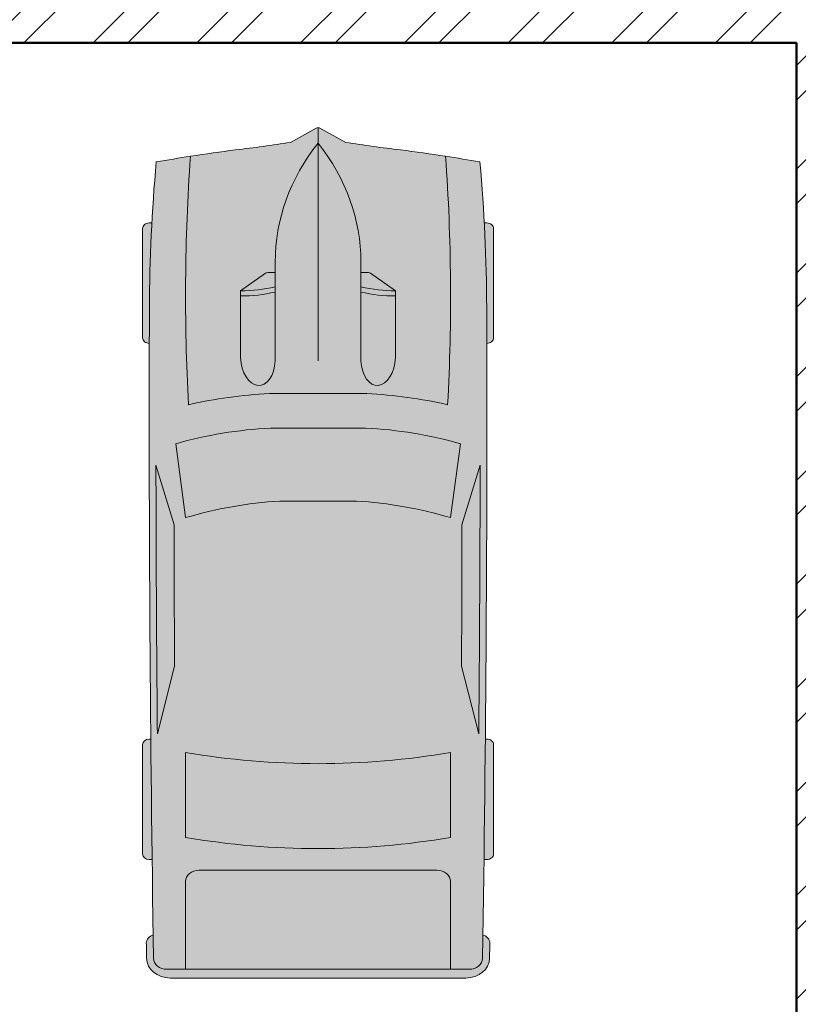
# Model space of a CAD drawing. Units: inches. Extents: x -31485 to -28799, y 18003 to 19130.
# Tile 2 of 15: x -30771 to -30670, y 18270 to 18398. Entities that reach past the tile are written whole.
import ezdxf

# ---------------------------------------------------------------- set-up
doc = ezdxf.new("R2010")
doc.units = ezdxf.units.IN
for name, color, linetype, lineweight in [('A-EQPM', 8, 'Continuous', 18), ('A-WALL', 7, 'Continuous', 50), ('A-WALL-PATT', 8, 'Continuous', 13)]:
    doc.layers.add(name, color=color, linetype=linetype, lineweight=lineweight)

# ---------------------------------------------------------------- blocks, each defined once
blk = doc.blocks.new('*U75')
for p, q in [((536.0433148737552, 950.1792138851854), (536.0433148737552, 935.5404748014407)), ((1182.463644577746, 987.7673041878503), (567.7039087844591, 987.7673041878503)), ((1214.124238488447, 949.7089586534819), (1214.124238488447, 950.1792138851854)), ((3440.463608272525, 941.6679440245914), (3440.463608272525, 950.1792138851854)), ((3472.124202183229, 987.7673041878503), (4086.88393797651, 987.767304187848)), ((4118.544531887212, 950.1792138851804), (4118.544531887212, 934.0601128753084)), ((2234.827175480885, 809.5287016048088), (1898.878785383111, 912.4126225124705)), ((3411.559256322833, 904.3494681924599), (3029.921878250559, 807.1504809911063)), ((4736.411271353851, -850.8646766016326), (4736.411271353883, 850.864676601626)), ((4785.334832293326, -832.0706314503777), (4785.334832293357, 832.0706314502926)), ((1778.76917512805, 801.0177247054045), (2194.716249451875, 745.5217224176465)), ((3515.941238262737, 745.5217224176508), (3994.062813016633, 745.5217224176508)), ((4736.411271353883, 745.5217224176529), (4242.012185201922, 745.5217224176529)), ((4178.690997380514, 670.345541812321), (4178.690997380509, -670.3455418123318)), ((819.5542361210883, 295.2827619512633), (917.6699264680983, 436.1082195367583)), ((917.6699264680983, 436.1082195367583), (1293.848362214069, 436.1082195367583)), ((815.9220749762081, 241.4481679439487), (815.9220749762081, 283.3039660446585)), ((756.2288711996046, 241.4481679439487), (1312.764151599097, 241.4481679439487)), ((1496.485716216861, -273.6820371142997), (1496.485716216861, 273.6820371142868)), ((1690.372337881975, -267.4332505757059), (1690.372337881975, 267.4332505756928)), ((4736.411271353883, -267.4332505757059), (4736.411271353883, 267.4332505756928)), ((2101.521373270556, 215.7994139342878), (2101.521373270556, -215.7994139342835)), ((82.96813941916749, 155.6585683733955), (2.596917328392246, 10.3141998552517)), ((-1.1252e-12, -6.4972e-12), (1312.764151599097, -6.4972e-12)), ((2.596917328392246, -10.31419985525964), (82.96813941916749, -155.6585683734063)), ((756.2288711996046, -241.4481679439617), (1312.764151599097, -241.4481679439617)), ((815.9220749762081, -241.4481679439617), (815.9220749762081, -283.3039660446715)), ((819.5542361210883, -295.2827619512763), (917.6699264680983, -436.1082195367712)), ((917.6699264680983, -436.1082195367712), (1293.848362214069, -436.1082195367712)), ((2194.716249451869, -745.5217224176688), (1778.769175128041, -801.0177247054262)), ((3994.062813016633, -745.5217224176616), (3515.941238262737, -745.5217224176638)), ((4242.012185201917, -745.5217224176638), (4736.411271353857, -745.5217224176594)), ((2234.827175480882, -809.5287016048153), (1898.878785383109, -912.4126225124726)), ((3411.559256322828, -904.349468192473), (3029.921878250557, -807.150480991115)), ((536.0433148737552, -950.1792138851984), (536.0433148737552, -935.5404748014537)), ((3440.463608272523, -941.6679440246044), (3440.463608272523, -950.1792138851984)), ((4118.544531887212, -950.1792138851933), (4118.544531887212, -934.0601128753214)), ((1182.463644577746, -987.7673041878633), (567.7039087844591, -987.7673041878633)), ((1214.124238488447, -949.7089586534948), (1214.124238488447, -950.1792138851984)), ((3472.124202183229, -987.7673041878633), (4086.883937976504, -987.767304187861))]:
    blk.add_line(p, q)
for centre, major_axis, ratio, start_param, end_param in [((1046.255263051279, -12467.92283887244), (3.2861e-12, 13417.14359589015), 0.8423038695439741, 0.0028100083536837, 0.0755983031096952), ((567.7039087844591, 950.1792138851861), (5.296e-13, -37.5880903026662), 0.842303869543976, 3.141592653589776, 4.712388980384677), ((1637.842620806017, -268112.68896731), (4.8454159e-09, 269062.8681811952), 0.842303869543847, -0.0133969486112073, 0.0027970409639888), ((1182.463644577746, 950.1792138851861), (5.601e-13, 37.58809030266621), 0.8423038695439758, -1.570796326794884, 1.73e-14), ((3472.124202183229, 950.1792138851861), (5.988e-12, -37.5880903026662), 0.8423038695439762, 3.141592653589603, 4.712388980384554), ((4086.88393797651, 950.179213885181), (1.4197e-12, 37.5880903026662), 0.842303869543976, -1.570796326794865, 4.44e-14), ((4587.952203166941, 910.2894362332722), (1.8792e-12, 56.38213545399769), 0.8423038695439691, -0.0130174256259048, 1.249894140392862), ((1637.84262086767, -268131.4830124673), (3.42859201765e-05, 269120.9512111412), 0.8423038681351471, -0.0133969484821159, -0.0130174254969711), ((4673.090083532448, 832.070631450172), (2.1733e-12, -133.2592106239272), 0.8423038695439737, 1.570796326795794, 3.128195704978164), ((6757.162543998887, -699.1204428451242), (4.9938223e-09, 7958.017136535005), 0.8423038695435286, 1.367075990158062, 1.391760499156098), ((1637.842620802809, -268112.6889680619), (4.87113144e-08, -269025.2800916445), 0.8423038695482963, 3.133765086725325, 3.140440689641252), ((4673.090083532475, 850.8646766015395), (7.5e-15, -75.17618060533067), 0.8423038695439952, 1.570796326796048, 3.128195704978389), ((3436.395912346701, 136.8410185571553), (5.76965e-11, 2077.023647078763), 0.8423038695439563, 1.245306111696802, 1.507880129813836), ((2433.035484508693, -93125.37499596032), (4.952654e-09, -93935.19844392464), 0.8423038695446962, 3.134048706297306, 3.14409775411291), ((951.8333444315502, -15086.63944974413), (1.5767e-12, -15832.53653317094), 0.8423038695439826, 3.09604606856106, 3.200911180495224), ((3413.769624379244, 136.8410185571329), (1.08602e-11, -2280.347340451234), 0.84230386954398, 4.44948196380473, 4.652344057257214), ((3799.722190048092, 71.1058404433382), (2.17448e-11, -2021.323467232052), 0.842303869543983, 4.372215489277867, 4.640744122441986), ((433.884764992104, -3.6096e-12), (1.7438e-12, 3734.255266801694), 0.8423038695439766, 4.511394369635731, 4.913383591133647), ((912.0063397460013, -3.6096e-12), (1.7438e-12, 3734.255266801694), 0.8423038695439766, 4.511394369635731, 4.913383591133647), ((4242.012185201922, 670.3455418123216), (3.5405e-12, 75.17618060533239), 0.842303869543976, 5.55e-14, 1.57079632679492), ((6583.045501169266, -699.1204428451198), (3.826807e-09, -7754.693443154298), 0.8423038695443791, 4.528606069860317, 4.561837674556238), ((-5194.164488957196, 1330.879982200552), (1.0466145e-09, -6374.389491984369), 0.8423038695441164, 1.385369446298923, 1.434372047871027), ((331.12799165183, 432.0470009052715), (3.125e-11, 696.3661584994836), 0.8423038695439277, 4.435146050259648, 4.718221029521873), ((360.7019022476185, 432.0470009052715), (3.125e-11, 696.3661584994836), 0.8423038695439277, 4.435146050259648, 4.718221029521873), ((1290.073045555822, 338.7781937403542), (161.0379696969085, -9.057857958340485), 0.6038335755719145, -1.39555193967809, 1.581314658479915), ((831.7523719315589, 283.3039660446593), (3.3347e-12, 18.79404515133458), 0.8423038695439091, 0.8797135699495516, 1.570796326795045), ((756.2288711996046, -1185.240851913765), (1.2998e-12, 1426.689019857713), 0.842303869543976, 7e-16, 0.5903187773915901), ((15.83029695535095, -3.6096e-12), (1.9e-15, -18.79404515133476), 0.842303869543842, 4.131459131953847, 5.293318828815531), ((756.2288711996046, 1185.240851913753), (1.01699e-11, 1426.689019857713), 0.8423038695439736, 2.55127387619821, 3.141592653589801), ((-5194.164488957196, -1330.879982200562), (1.0234792e-09, 6374.389491984348), 0.8423038695441192, -1.43437204787103, -1.385369446298926), ((3799.722190048497, -71.10584044329416), (1.038796e-10, -2021.323467232635), 0.8423038695439419, -1.499151468852248, -1.230622835688196), ((331.12799165183, -432.0470009052816), (3.1922e-11, -696.3661584994801), 0.842303869543932, 1.564964277657711, 1.848039256919935), ((360.7019022476185, -432.0470009052816), (3.1922e-11, -696.3661584994801), 0.842303869543932, 1.564964277657711, 1.848039256919935), ((3413.769624379237, -136.841018557156), (1.090899e-10, -2280.347340451348), 0.8423038695439354, -1.510751403667474, -1.307889310215002), ((3436.395912346742, -136.8410185572101), (8.13766e-11, -2077.023647078826), 0.8423038695439492, -1.50788012981387, -1.245306111696839), ((831.7523719315589, -283.3039660446737), (3.3028e-12, -18.79404515133458), 0.8423038695439093, 4.712388980384541, 5.403471737230034), ((6583.045501169163, 699.1204428449458), (2.756795e-10, 7754.693443157768), 0.8423038695439974, 1.721347632622872, 1.754579237318777), ((6757.162543998887, 699.1204428451076), (2.2231118e-09, 7958.017136528592), 0.8423038695441819, 1.749832154434603, 1.774516663432659), ((951.8333444315729, 15086.63944974408), (2.97009e-11, -15832.5365331709), 0.8423038695439528, -0.0593185269054384, 0.0455465850287298), ((4242.012185201917, -670.3455418123318), (2.579e-13, -75.17618060533128), 0.8423038695439885, 4.712388980384686, 6.283185307179581), ((2433.03548450906, 93125.37499596029), (4.1600574e-09, -93935.19844392457), 0.8423038695447548, -0.0025051005232382, 0.007543947292366), ((4673.090083532448, -850.8646766015358), (2.354e-13, 75.17618060532999), 0.8423038695439732, 3.154989602201626, 4.71238898038339), ((4673.090083532349, -832.0706314501077), (6.1679e-12, -133.2592106240062), 0.8423038695439807, 0.0133969486110846, 1.570796326792831), ((1046.255263051284, 12467.92283887242), (3.49903e-10, -13417.14359589015), 0.8423038695440652, -0.0755983031097181, -0.0028100083537155), ((1637.842620801787, 268112.6889680619), (1.55395844e-08, 269062.868181947), 0.8423038695458147, 3.138795612625926, 3.154989602201039), ((1637.842620803916, 268112.6889680615), (4.0766478e-08, -269025.280091644), 0.8423038695397146, 0.0011519639481523, 0.0078275668641468), ((4587.952203166856, -910.2894362333229), (5.777e-12, -56.38213545402103), 0.8423038695439803, -1.249894138785958, 0.0130174256254374), ((567.7039087844591, -950.1792138851977), (5.601e-13, 37.58809030266621), 0.8423038695439758, 1.570796326794908, 3.14159265358981), ((1182.463644577746, -950.1792138851977), (5.296e-13, -37.5880903026662), 0.842303869543976, -1.69e-14, 1.570796326794884), ((3472.124202183229, -950.1792138851955), (3.96e-13, -37.58809030266733), 0.8423038695440105, -1.570796326794875, -1.27e-14), ((4086.883937976504, -950.1792138851933), (5.0003e-12, 37.58809030266732), 0.8423038695440109, 3.141592653589951, 4.712388980384771), ((1637.842620726191, 268131.4830135791), (2.37878358395e-05, 269120.9512123862), 0.8423038705260315, 3.154610079306566, 3.154989602290631)]:
    blk.add_ellipse(centre, major_axis=major_axis, ratio=ratio, start_param=start_param, end_param=end_param)
at = {"extrusion": (0, 0, -1)}
blk.add_ellipse((1290.073045555822, -338.7781937403665), major_axis=(161.0379696969085, 9.057857958340424), ratio=0.6038335755719145, start_param=-1.39555193967809, end_param=1.581314658479915, dxfattribs=at)

msp = doc.modelspace()

# ---------------------------------------------------------------- hatches: boundary and pattern name
at = {"layer": 'A-EQPM'}
h = msp.add_hatch(color=256, dxfattribs=at)
h.dxf.hatch_style = 1
edge = h.paths.add_edge_path()
edge.add_ellipse((-30729.51109539866, 18304.50617737439), major_axis=(-47.91849192778267, 1.361529e-10), ratio=0.8423038695419347, start_angle=248.1650462034528, end_angle=265.722579037107)
edge.add_line((-30726.49823474847, 18344.78824959643), (-30738.838005725, 18344.78824959643))
edge.add_ellipse((-30735.82514507481, 18304.50617737439), major_axis=(47.91849192778146, 1.460375e-10), ratio=0.8423038695419556, start_angle=94.277420962876, end_angle=111.8349537965306)
edge.add_line((-30751.14819937748, 18342.74886832219), (-30749.86786501952, 18333.15265763323))
edge.add_ellipse((-30734.30858525796, 18296.12396789418), major_axis=(46.63344704056234, 1.445442e-10), ratio=0.842303869541784, start_angle=94.8700695969602, end_angle=112.7919148774121, ccw=False)
edge.add_line((-30737.64677442257, 18335.30273326105), (-30727.6894660509, 18335.30273326105))
edge.add_ellipse((-30731.02765521551, 18296.12396789419), major_axis=(-46.63344704055716, 1.546607e-10), ratio=0.8423038695417213, start_angle=247.20808512260112, end_angle=265.1299304030565, ccw=False)
edge.add_line((-30715.46837545394, 18333.15265763323), (-30714.18804109599, 18342.74886832219))
edge = h.paths.add_edge_path()
edge.add_ellipse((-30760.01251483457, 18366.33963936055), major_axis=(-32.91478475822442, 2.78257e-11), ratio=0.8423038695443898, start_angle=180.0000000000484, end_angle=209.4385695980319)
edge.add_ellipse((-30705.3237256389, 18366.33963936055), major_axis=(32.91478475822442, 2.78184e-11), ratio=0.8423038695443903, start_angle=150.561430401968, end_angle=179.9999999999515)
edge.add_line((-30738.23851039712, 18366.33963936055), (-30738.23851039712, 18353.49995340956))
edge.add_ellipse((-30740.48398702518, 18354.02345422925), major_axis=(-0.2089715704820894, 3.715266632531377), ratio=0.6038335755718302, start_angle=89.0020142750023, end_angle=253.6574080457279, ccw=False)
edge.add_line((-30742.72946365324, 18353.93635484496), (-30742.72946365324, 18362.61507324184))
edge.add_line((-30742.72946365324, 18362.61507324184), (-30739.40197717196, 18364.93339436665))
edge.add_ellipse((-30739.20415502338, 18364.59725560616), major_axis=(0.4335927047225755, 4.12191e-11), ratio=0.8423038695061222, start_angle=89.99999999455332, end_angle=134.4802108771379, ccw=False)
edge.add_line((-30739.20415502338, 18364.96247241913), (-30738.23851039712, 18364.96247241913))
edge.add_line((-30738.23851039712, 18364.96247241913), (-30738.23851039712, 18366.33963936055))
edge.add_ellipse((-30705.3237256389, 18366.33963936055), major_axis=(32.91478475822442, 2.78184e-11), ratio=0.8423038695443903, start_angle=150.5614304019681, end_angle=179.9999999999516, ccw=False)
edge.add_line((-30732.66812023673, 18381.77167472263), (-30732.66812023673, 18383.786406089))
edge.add_ellipse((-30732.66812023673, 18383.42118927602), major_axis=(-0.4335927046986816, 0), ratio=0.842303869552539, start_angle=270, end_angle=307.9331304600232)
edge.add_line((-30732.9060765562, 18383.72649326027), (-30736.25928004974, 18381.87226894154))
edge.add_ellipse((-30763.372518703, 18503.6196730261), major_axis=(-147.0619421372835, 4.9907306e-09), ratio=0.8423038695736066, start_angle=99.2565660091451, end_angle=102.55493264608151, ccw=False)
edge.add_ellipse((-30716.53888774386, 18231.91061346098), major_axis=(178.9065886092977, 1.2789651e-09), ratio=0.8423038695391513, start_angle=100.209538996733, end_angle=102.4446272930335)
edge.add_ellipse((-30384.60804316206, 18361.82689758953), major_axis=(365.2684817172171, 7.18011e-11), ratio=0.8423038695434502, start_angle=177.1362853921513, end_angle=182.1985405659441)
edge.add_ellipse((-30735.82514507481, 18305.0281827925), major_axis=(52.60932189168197, 7.16232e-11), ratio=0.8423038695431074, start_angle=94.08241069107589, end_angle=107.71995322267611, ccw=False)
edge.add_line((-30738.98216991289, 18349.26135924456), (-30726.35407056058, 18349.26135924456))
edge.add_ellipse((-30729.51109539866, 18305.0281827925), major_axis=(-52.6093218916263, 2.96862e-11), ratio=0.842303869543985, start_angle=252.2800467772827, end_angle=265.9175893088832, ccw=False)
edge.add_ellipse((-31080.72819731141, 18361.82689758953), major_axis=(365.2684817172168, 5.54988e-11), ratio=0.8423038695419378, start_angle=-2.198540565964143, end_angle=2.863714607828726)
edge.add_ellipse((-30748.79735272961, 18231.91061346097), major_axis=(-178.9065886093012, 1.2581094e-09), ratio=0.8423038695391548, start_angle=257.5553727069574, end_angle=259.7904610032577)
edge.add_ellipse((-30701.96372177047, 18503.6196730261), major_axis=(147.0619421407358, 1.9919546e-09), ratio=0.8423038695542743, start_angle=257.4450673550873, end_angle=260.74343399202326, ccw=False)
edge.add_line((-30729.07696042372, 18381.87226894154), (-30732.43016391727, 18383.72649326027))
edge.add_ellipse((-30732.66812023673, 18383.42118927602), major_axis=(-0.4335927046986816, 0), ratio=0.842303869552539, start_angle=232.0668695399768, end_angle=270)
edge.add_line((-30732.66812023673, 18383.786406089), (-30732.66812023673, 18381.77167472263))
edge.add_ellipse((-30760.01251483457, 18366.33963936055), major_axis=(-32.91478475822442, 2.78257e-11), ratio=0.8423038695443898, start_angle=180.0000000000485, end_angle=209.438569598032, ccw=False)
edge.add_line((-30727.09773007635, 18366.33963936055), (-30727.09773007635, 18364.96247241913))
edge.add_line((-30727.09773007635, 18364.96247241913), (-30725.97599903238, 18364.96247241913))
edge.add_line((-30725.97599903238, 18364.96247241913), (-30722.60677682023, 18362.61507324184))
edge.add_line((-30722.60677682023, 18362.61507324184), (-30722.60677682023, 18353.93635484496))
edge.add_ellipse((-30724.85225344829, 18354.02345422925), major_axis=(0.2089715704820894, 3.715266632531377), ratio=0.6038335755718302, start_angle=106.3425919542722, end_angle=270.9979857249977, ccw=False)
edge.add_line((-30727.09773007635, 18353.49995340956), (-30727.09773007635, 18366.33963936055))
edge = h.paths.add_edge_path()
edge.add_ellipse((-28584.1959368406, 18327.65445429916), major_axis=(-2167.155417170912, 9.004676e-10), ratio=0.8423038695746358, start_angle=-0.12089736900918524, end_angle=0.3640763489138976, ccw=False)
edge.add_line((-30751.34455399213, 18332.22726851316), (-30753.71816314214, 18339.97784961109))
edge.add_ellipse((-24547.10747912888, 18346.00014953185), major_axis=(6206.614802166701, 5.2511138e-09), ratio=0.842303869515611, start_angle=180.0555943134505, end_angle=180.377764193861)
edge.add_line((-30753.53214012996, 18305.07917763989), (-30751.28968666049, 18313.88383792681))
edge = h.paths.add_edge_path()
edge.add_ellipse((-36918.2287613446, 18346.00014953188), major_axis=(-6206.61480216671, 6.192387e-09), ratio=0.8423038695127218, start_angle=179.6222358061472, end_angle=179.9444056865578)
edge.add_line((-30711.61807733132, 18339.97784961108), (-30713.99168648134, 18332.22726851316))
edge.add_ellipse((-32881.14030363287, 18327.65445429917), major_axis=(-2167.155417170919, 1.3253717e-09), ratio=0.8423038695188795, start_angle=179.6359236511448, end_angle=180.1208973690678, ccw=False)
edge.add_line((-30714.04655381298, 18313.88383792681), (-30711.8041003435, 18305.07917763988))
edge = h.paths.add_edge_path()
edge.add_ellipse((-30732.66812023673, 18373.77635943495), major_axis=(-86.15206721880882, 2.44e-14), ratio=0.8423038695434939, start_angle=76.40186530976911, end_angle=103.598134690231, ccw=False)
edge.add_line((-30749.86786501952, 18302.67100709929), (-30749.86786501952, 18291.64038409579))
edge.add_ellipse((-30732.66812023673, 18362.74573643145), major_axis=(-86.15206721880666, 5.3e-15), ratio=0.8423038695434728, start_angle=76.40186530976838, end_angle=103.5981346902316)
edge.add_line((-30715.46837545394, 18291.64038409579), (-30715.46837545394, 18302.67100709929))
edge = h.paths.add_edge_path()
edge.add_ellipse((-30717.20274627276, 18285.92000628197), major_axis=(-1.734370818820025, 1.15572e-11), ratio=0.8423038695444475, start_angle=180.0000000003817, end_angle=270.0000000003818)
edge.add_line((-30717.20274627276, 18287.38087353389), (-30748.1334942007, 18287.38087353389))
edge.add_ellipse((-30748.1334942007, 18285.92000628197), major_axis=(1.734370818820025, 1.15576e-11), ratio=0.8423038695444475, start_angle=89.99999999961817, end_angle=179.9999999996181)
edge.add_line((-30749.86786501952, 18285.92000628197), (-30749.86786501952, 18274.51384889318))
edge.add_line((-30749.86786501952, 18274.51384889318), (-30715.46837545394, 18274.51384889318))
edge.add_line((-30715.46837545394, 18274.51384889318), (-30715.46837545394, 18285.92000628197))
h = msp.add_hatch(color=256, dxfattribs=at)
h.dxf.hatch_style = 1
edge = h.paths.add_edge_path()
edge.add_ellipse((-36918.22876132725, 18346.0001495318), major_axis=(6207.481987558777, 4.152598e-10), ratio=0.8423038695472291, start_angle=-0.3838667787963557, end_angle=0.0902290885904627)
edge.add_ellipse((-36918.22876132725, 18346.0001495318), major_axis=(6207.481987558777, 4.152598e-10), ratio=0.8423038695472291, start_angle=0.0902290885904627, end_angle=0.1349865768543979)
edge.add_ellipse((-31020.31244279875, 18359.64851317319), major_axis=(309.5435567121417, 3.12922e-11), ratio=0.8423038695440732, start_angle=0.1806905311799308, end_angle=2.179950313639523)
edge.add_ellipse((-31020.31244279875, 18359.64851317319), major_axis=(309.5435567121417, 3.12922e-11), ratio=0.8423038695440732, start_angle=2.179950313639523, end_angle=3.650427585692763)
edge.add_ellipse((-30748.79735272961, 18227.89360281064), major_axis=(183.5974185536168, 2.07254122e-08), ratio=0.8423038696260594, start_angle=76.2194710040335, end_angle=77.87403444124779)
edge.add_ellipse((-31080.72819731141, 18361.82689758953), major_axis=(365.2684817172168, 5.54988e-11), ratio=0.8423038695419378, start_angle=-2.1985405659640946, end_angle=2.8637146078286833, ccw=False)
edge.add_ellipse((-30729.51109539866, 18305.0281827925), major_axis=(-52.6093218916263, 2.96862e-11), ratio=0.842303869543985, start_angle=252.2800467772827, end_angle=265.9175893088831)
edge.add_line((-30726.35407056058, 18349.26135924456), (-30738.98216991289, 18349.26135924456))
edge.add_ellipse((-30735.82514507481, 18305.0281827925), major_axis=(52.60932189168197, 7.16232e-11), ratio=0.8423038695431074, start_angle=94.08241069107586, end_angle=107.719953222676)
edge.add_ellipse((-30384.60804316206, 18361.82689758953), major_axis=(365.2684817172171, 7.18011e-11), ratio=0.8423038695434502, start_angle=177.1362853921513, end_angle=182.1985405659441, ccw=False)
edge.add_ellipse((-30716.53888774386, 18227.89360281064), major_axis=(-183.5974185535601, 2.07797544e-08), ratio=0.8423038696263095, start_angle=-77.87403444123211, end_angle=-76.21947100401783)
edge.add_ellipse((-30445.02379767472, 18359.64851317319), major_axis=(-309.5435567121417, 3.20483e-11), ratio=0.8423038695440663, start_angle=-3.650427585692615, end_angle=-2.179950313639383)
edge.add_ellipse((-30445.02379767472, 18359.64851317319), major_axis=(-309.5435567121417, 3.20483e-11), ratio=0.8423038695440663, start_angle=-2.179950313639383, end_angle=-0.1356123904320413)
edge.add_ellipse((-24547.10747912888, 18346.0001495319), major_axis=(6207.481987576122, 7.89454e-11), ratio=0.842303869542251, start_angle=179.8650134231422, end_angle=179.9097709114061)
edge.add_ellipse((-24547.10747912888, 18346.0001495319), major_axis=(6207.481987576122, 7.89454e-11), ratio=0.842303869542251, start_angle=179.9097709114061, end_angle=180.3838667787915)
edge.add_ellipse((-24547.10747912888, 18346.0001495319), major_axis=(6207.481987576122, 7.89454e-11), ratio=0.842303869542251, start_angle=180.3838667787915, end_angle=180.5282714718166)
edge.add_ellipse((-24547.10747912888, 18346.0001495319), major_axis=(6207.481987576122, 7.89454e-11), ratio=0.842303869542251, start_angle=180.5282714718166, end_angle=180.6465540970602)
edge.add_ellipse((-30752.29820590986, 18275.9747161451), major_axis=(1.734370818820398, 6.2835e-12), ratio=0.8423038695442665, start_angle=180.6465540968934, end_angle=269.9999999996497)
edge.add_line((-30752.29820590986, 18274.51384889318), (-30749.86786501952, 18274.51384889318))
edge.add_line((-30749.86786501952, 18274.51384889318), (-30749.86786501952, 18286.45472080772))
edge.add_ellipse((-30748.1334942007, 18285.92000628197), major_axis=(1.734370818820025, 1.15576e-11), ratio=0.8423038695444475, start_angle=89.99999999961818, end_angle=179.9999999996182, ccw=False)
edge.add_line((-30748.1334942007, 18287.38087353389), (-30716.5679224935, 18287.38087353389))
edge.add_ellipse((-30717.20274627276, 18285.92000628197), major_axis=(-1.734370818820025, 1.15572e-11), ratio=0.8423038695444475, start_angle=180.0000000003818, end_angle=270.00000000038176, ccw=False)
edge.add_line((-30715.46837545394, 18285.92000628197), (-30715.46837545394, 18274.51384889318))
edge.add_line((-30715.46837545394, 18274.51384889318), (-30713.0380345636, 18274.51384889318))
edge.add_ellipse((-30713.03803456361, 18275.9747161451), major_axis=(-1.734370818820364, 1.2413e-12), ratio=0.8423038695421853, start_angle=90.00000000018369, end_angle=179.3534459030602)
edge.add_ellipse((-36918.22876132725, 18346.0001495318), major_axis=(6207.481987558777, 4.152598e-10), ratio=0.8423038695472291, start_angle=-0.6465540970657812, end_angle=-0.618643196323059)
edge.add_ellipse((-36918.22876132725, 18346.0001495318), major_axis=(6207.481987558777, 4.152598e-10), ratio=0.8423038695472291, start_angle=-0.618643196323059, end_angle=-0.528271471821792)
edge.add_ellipse((-36918.22876132725, 18346.0001495318), major_axis=(6207.481987558777, 4.152598e-10), ratio=0.8423038695472291, start_angle=-0.528271471821792, end_angle=-0.3838667787963557)
edge = h.paths.add_edge_path(flags=16)
edge.add_ellipse((-30734.30858525796, 18296.12396789418), major_axis=(46.63344704056234, 1.445442e-10), ratio=0.842303869541784, start_angle=94.8700695969603, end_angle=112.7919148774121)
edge.add_line((-30749.86786501952, 18333.15265763323), (-30751.14819937748, 18342.74886832219))
edge.add_ellipse((-30735.82514507481, 18304.50617737439), major_axis=(47.91849192778146, 1.460375e-10), ratio=0.8423038695419556, start_angle=94.27742096287608, end_angle=111.8349537965307, ccw=False)
edge.add_line((-30738.838005725, 18344.78824959643), (-30726.49823474847, 18344.78824959643))
edge.add_ellipse((-30729.51109539866, 18304.50617737439), major_axis=(-47.91849192778267, 1.361529e-10), ratio=0.8423038695419347, start_angle=248.1650462034528, end_angle=265.72257903710704, ccw=False)
edge.add_line((-30714.18804109599, 18342.74886832219), (-30715.46837545394, 18333.15265763323))
edge.add_ellipse((-30731.02765521551, 18296.12396789419), major_axis=(-46.63344704055716, 1.546607e-10), ratio=0.8423038695417213, start_angle=247.208085122601, end_angle=265.1299304030565)
edge.add_line((-30727.6894660509, 18335.30273326105), (-30737.64677442257, 18335.30273326105))
edge = h.paths.add_edge_path(flags=16)
edge.add_line((-30713.99168648134, 18332.22726851316), (-30711.61807733132, 18339.97784961108))
edge.add_ellipse((-36918.2287613446, 18346.00014953188), major_axis=(-6206.61480216671, 6.192387e-09), ratio=0.8423038695127218, start_angle=179.6222358061473, end_angle=179.9444056865578, ccw=False)
edge.add_line((-30711.8041003435, 18305.07917763988), (-30714.04655381298, 18313.88383792681))
edge.add_ellipse((-32881.14030363287, 18327.65445429917), major_axis=(-2167.155417170919, 1.3253717e-09), ratio=0.8423038695188795, start_angle=179.6359236511447, end_angle=180.1208973690677)
edge = h.paths.add_edge_path(flags=16)
edge.add_ellipse((-28584.1959368406, 18327.65445429916), major_axis=(-2167.155417170912, 9.004676e-10), ratio=0.8423038695746358, start_angle=-0.1208973690091865, end_angle=0.364076348913875)
edge.add_line((-30751.28968666049, 18313.88383792681), (-30753.53214012996, 18305.07917763989))
edge.add_ellipse((-24547.10747912888, 18346.00014953185), major_axis=(6206.614802166701, 5.2511138e-09), ratio=0.842303869515611, start_angle=180.0555943134506, end_angle=180.3777641938611, ccw=False)
edge.add_line((-30753.71816314214, 18339.97784961109), (-30751.34455399213, 18332.22726851316))
edge = h.paths.add_edge_path(flags=16)
edge.add_ellipse((-30732.66812023673, 18373.77635943495), major_axis=(-86.15206721880882, 2.44e-14), ratio=0.8423038695434939, start_angle=76.40186530976904, end_angle=103.5981346902309)
edge.add_line((-30715.46837545394, 18302.67100709929), (-30715.46837545394, 18291.64038409579))
edge.add_ellipse((-30732.66812023673, 18362.74573643145), major_axis=(-86.15206721880666, 5.3e-15), ratio=0.8423038695434728, start_angle=76.40186530976843, end_angle=103.59813469023157, ccw=False)
edge.add_line((-30749.86786501952, 18291.64038409579), (-30749.86786501952, 18302.67100709929))
h = msp.add_hatch(color=256, dxfattribs=at)
h.dxf.hatch_style = 1
edge = h.paths.add_edge_path()
edge.add_ellipse((-30722.70047217728, 18376.14703519531), major_axis=(-16.06568908915088, 3.60949e-11), ratio=0.8423038695435023, start_angle=71.33250450753093, end_angle=90.39670986011208, ccw=False)
edge.add_line((-30727.09773007635, 18363.13158723229), (-30727.09773007635, 18362.44929495403))
edge.add_ellipse((-30722.70047217728, 18375.46474291706), major_axis=(16.06568908904641, 9.1463e-11), ratio=0.8423038695487669, start_angle=251.332504507076, end_angle=270.3967098596572)
edge.add_line((-30722.60677682023, 18361.93278096359), (-30722.60677682023, 18362.61507324184))
edge = h.paths.add_edge_path()
edge.add_ellipse((-30742.63576829619, 18376.14703519531), major_axis=(16.06568908915091, 3.60949e-11), ratio=0.8423038695435009, start_angle=269.6032901398879, end_angle=288.667495492469, ccw=False)
edge.add_line((-30742.72946365324, 18362.61507324184), (-30742.72946365324, 18361.93278096359))
edge.add_ellipse((-30742.63576829619, 18375.46474291706), major_axis=(-16.06568908904639, 9.1463e-11), ratio=0.8423038695487673, start_angle=89.60329014034272, end_angle=108.667495492924)
edge.add_line((-30738.23851039712, 18362.44929495403), (-30738.23851039712, 18363.13158723229))
edge = h.paths.add_edge_path()
edge.add_ellipse((-30710.74677376847, 18370.6890515121), major_axis=(0.8671854094100124, 1.6795e-12), ratio=0.8423038695444477, start_angle=-1.109639e-10, end_angle=89.99999999988906)
edge.add_line((-30710.74677376847, 18371.41948513806), (-30711.08450044847, 18371.41948513806))
edge.add_ellipse((-31020.31244279875, 18359.64851317319), major_axis=(309.5435567121417, 3.12922e-11), ratio=0.8423038695440732, start_angle=0.18069053117989142, end_angle=2.1799503136394947, ccw=False)
edge.add_ellipse((-31020.31244279875, 18359.64851317319), major_axis=(309.5435567121417, 3.12922e-11), ratio=0.8423038695440732, start_angle=0.1356123904321862, end_angle=0.18069053117989142, ccw=False)
edge.add_ellipse((-36918.22876132725, 18346.0001495318), major_axis=(6207.481987558777, 4.152598e-10), ratio=0.8423038695472291, start_angle=0.09022908859049039, end_angle=0.13498657685437365, ccw=False)
edge.add_line((-30710.75762290904, 18355.7756501195), (-30710.74677376847, 18355.7756501195))
edge.add_ellipse((-30710.74677376847, 18356.50608374546), major_axis=(-0.8671854094100128, 1.6795e-12), ratio=0.8423038695444475, start_angle=90.00000000011094, end_angle=180.0000000001109)
edge.add_line((-30709.87958835906, 18356.50608374546), (-30709.87958835906, 18370.6890515121))
edge = h.paths.add_edge_path()
edge.add_ellipse((-30445.02379767472, 18359.64851317319), major_axis=(-309.5435567121417, 3.20483e-11), ratio=0.8423038695440663, start_angle=-2.179950313639381, end_angle=-0.13561239043201567, ccw=False)
edge.add_line((-30754.251740025, 18371.41948513806), (-30754.589466705, 18371.41948513806))
edge.add_ellipse((-30754.589466705, 18370.6890515121), major_axis=(-0.8671854094100128, 1.6795e-12), ratio=0.8423038695444475, start_angle=-89.99999999988903, end_angle=1.109639e-10)
edge.add_line((-30755.45665211441, 18370.6890515121), (-30755.45665211441, 18356.50608374546))
edge.add_ellipse((-30754.589466705, 18356.50608374546), major_axis=(0.8671854094100124, 1.6795e-12), ratio=0.8423038695444477, start_angle=179.999999999889, end_angle=269.999999999889)
edge.add_line((-30754.589466705, 18355.7756501195), (-30754.57861756442, 18355.7756501195))
edge.add_ellipse((-24547.10747912888, 18346.0001495319), major_axis=(6207.481987576122, 7.89454e-11), ratio=0.842303869542251, start_angle=179.8650134231423, end_angle=179.9097709114062, ccw=False)
edge = h.paths.add_edge_path()
edge.add_ellipse((-30713.47162726831, 18275.9747161451), major_axis=(3.074389845080431, 4.5193e-12), ratio=0.8423038695441155, start_angle=269.9999999999962, end_angle=359.3534459027799)
edge.add_ellipse((-36918.66235403209, 18346.00014953038), major_axis=(6208.822006597157, 5.2733581016e-06), ratio=0.8423038788855699, start_angle=-0.6465541457119849, end_angle=-0.6282372648788389)
edge.add_ellipse((-30711.66706082976, 18277.93891084205), major_axis=(-1.30077811411332, 2.65586e-11), ratio=0.8423038695457158, start_angle=179.3717627849924, end_angle=248.4647566023133)
edge.add_ellipse((-36918.22876132725, 18346.0001495318), major_axis=(6207.481987558777, 4.152598e-10), ratio=0.8423038695472291, start_angle=-0.6465540970658026, end_angle=-0.6186431963230916, ccw=False)
edge.add_ellipse((-30713.03803456361, 18275.9747161451), major_axis=(-1.734370818820364, 1.2413e-12), ratio=0.8423038695421853, start_angle=90.00000000018372, end_angle=179.3534459030602, ccw=False)
edge.add_line((-30713.0380345636, 18274.51384889318), (-30752.29820590986, 18274.51384889318))
edge.add_ellipse((-30752.29820590986, 18275.9747161451), major_axis=(1.734370818820398, 6.2835e-12), ratio=0.8423038695442665, start_angle=180.6465540968934, end_angle=269.99999999964973, ccw=False)
edge.add_ellipse((-24547.10747912888, 18346.0001495319), major_axis=(6207.481987576122, 7.89454e-11), ratio=0.842303869542251, start_angle=180.5282714718167, end_angle=180.6465540970602, ccw=False)
edge.add_ellipse((-30753.66917964371, 18277.93891084205), major_axis=(1.300778114113422, 3.7711e-12), ratio=0.8423038695465029, start_angle=111.5352435038071, end_angle=180.6282372160113)
edge.add_ellipse((-24546.67388641573, 18346.00014953364), major_axis=(-6208.822006624284, 5.909233014e-06), ratio=0.842303880027109, start_angle=0.6282372707742053, end_angle=0.6465541516072572)
edge.add_ellipse((-30751.86461320515, 18275.9747161451), major_axis=(-3.074389845084005, 2.9376e-12), ratio=0.8423038695431365, start_angle=0.6465540971220629, end_angle=89.99999999989375)
edge.add_line((-30751.86461320516, 18273.3851456821), (-30713.47162726831, 18273.3851456821))
edge = h.paths.add_edge_path()
edge.add_ellipse((-24547.10747912888, 18346.0001495319), major_axis=(6207.481987576122, 7.89454e-11), ratio=0.842303869542251, start_angle=180.3838667787916, end_angle=180.5282714718167, ccw=False)
edge.add_line((-30754.39310533151, 18304.41233258131), (-30754.589466705, 18304.41233258131))
edge.add_ellipse((-30754.589466705, 18303.68189895535), major_axis=(-0.8671854094100128, 1.6795e-12), ratio=0.8423038695444475, start_angle=-89.99999999988903, end_angle=1.109639e-10)
edge.add_line((-30755.45665211441, 18303.68189895535), (-30755.45665211441, 18289.49893118871))
edge.add_ellipse((-30754.589466705, 18289.49893118871), major_axis=(-0.8671854094100128, 3.5068e-12), ratio=0.8423038695402523, start_angle=2.317008e-10, end_angle=90.0000000002317)
edge.add_line((-30754.589466705, 18288.76849756276), (-30754.21758696607, 18288.76849756276))
edge = h.paths.add_edge_path()
edge.add_ellipse((-30710.74677376847, 18303.68189895535), major_axis=(0.8671854094100124, 1.6795e-12), ratio=0.8423038695444477, start_angle=-1.109639e-10, end_angle=89.99999999988906)
edge.add_line((-30710.74677376847, 18304.41233258131), (-30710.94313514195, 18304.41233258131))
edge.add_ellipse((-36918.22876132725, 18346.0001495318), major_axis=(6207.481987558777, 4.152598e-10), ratio=0.8423038695472291, start_angle=-0.5282714718218244, end_angle=-0.38386677879640274, ccw=False)
edge.add_line((-30711.1186535074, 18288.76849756276), (-30710.74677376847, 18288.76849756276))
edge.add_ellipse((-30710.74677376847, 18289.49893118871), major_axis=(0.8671854094100124, 3.5068e-12), ratio=0.8423038695402528, start_angle=269.9999999997683, end_angle=359.9999999997682)
edge.add_line((-30709.87958835906, 18289.49893118871), (-30709.87958835906, 18303.68189895535))
h = msp.add_hatch(color=256, dxfattribs=at)
h.dxf.hatch_style = 1
edge = h.paths.add_edge_path()
edge.add_ellipse((-30722.70047217728, 18375.46474291706), major_axis=(16.06568908904641, 9.1463e-11), ratio=0.8423038695487669, start_angle=251.332504507076, end_angle=270.3967098596572, ccw=False)
edge.add_line((-30727.09773007635, 18362.44929495403), (-30727.09773007635, 18353.49995340956))
edge.add_ellipse((-30724.85225344829, 18354.02345422925), major_axis=(0.2089715704820894, 3.715266632531377), ratio=0.6038335755718302, start_angle=106.3425919542721, end_angle=270.9979857249977)
edge.add_line((-30722.60677682023, 18353.93635484496), (-30722.60677682023, 18361.93278096359))
edge = h.paths.add_edge_path()
edge.add_line((-30738.23851039712, 18364.96247241913), (-30739.20415502338, 18364.96247241913))
edge.add_ellipse((-30739.20415502338, 18364.59725560616), major_axis=(0.4335927047225755, 4.12191e-11), ratio=0.8423038695061222, start_angle=89.99999999455322, end_angle=134.4802108771379)
edge.add_line((-30739.48051482109, 18364.87867573981), (-30742.72946365324, 18362.61507324184))
edge.add_ellipse((-30742.63576829619, 18376.14703519531), major_axis=(16.06568908915091, 3.60949e-11), ratio=0.8423038695435009, start_angle=269.6032901398879, end_angle=288.6674954924691)
edge.add_line((-30738.23851039712, 18363.13158723229), (-30738.23851039712, 18364.96247241913))
edge = h.paths.add_edge_path()
edge.add_ellipse((-30742.63576829619, 18375.46474291706), major_axis=(-16.06568908904639, 9.1463e-11), ratio=0.8423038695487673, start_angle=89.60329014034278, end_angle=108.66749549292399, ccw=False)
edge.add_line((-30742.72946365324, 18361.93278096359), (-30742.72946365324, 18353.93635484496))
edge.add_ellipse((-30740.48398702518, 18354.02345422925), major_axis=(-0.2089715704820894, 3.715266632531377), ratio=0.6038335755718302, start_angle=89.00201427500228, end_angle=253.6574080457278)
edge.add_line((-30738.23851039712, 18353.49995340956), (-30738.23851039712, 18362.44929495403))
edge = h.paths.add_edge_path()
edge.add_ellipse((-30726.13208545009, 18364.59725560616), major_axis=(-0.4335927047225754, 4.1219e-11), ratio=0.8423038695061223, start_angle=225.5197891228621, end_angle=270.0000000054467)
edge.add_line((-30726.13208545009, 18364.96247241913), (-30727.09773007635, 18364.96247241913))
edge.add_line((-30727.09773007635, 18364.96247241913), (-30727.09773007635, 18363.13158723229))
edge.add_ellipse((-30722.70047217728, 18376.14703519531), major_axis=(-16.06568908915088, 3.60949e-11), ratio=0.8423038695435023, start_angle=71.33250450753091, end_angle=90.39670986011207)
edge.add_line((-30722.60677682023, 18362.61507324184), (-30725.85572565238, 18364.87867573981))
at = {"layer": 'A-WALL-PATT'}
h = msp.add_hatch(dxfattribs=at)
h.set_pattern_fill('ANSI32', color=256)
h.set_pattern_definition([(45, (-1687.357050595019, -0.3129728357926069), (-6.735192090801865, 6.735192090801866), []), (45, (-1682.866920595021, -0.3129728357926069), (-6.735192090801865, 6.735192090801866), [])])
h.paths.add_polyline_path([(-31156.52828769349, 18823.80296009311), (-31209.52828769349, 18823.80296009311), (-31209.52828769349, 18761.80296009311), (-31200.52828769349, 18761.80296009311), (-31200.52828769349, 18814.80296009311), (-31156.52828769349, 18814.80296009311)], flags=17)
h.paths.add_polyline_path([(-31022.5282876935, 18823.80296009311), (-31118.52828769349, 18823.80296009311), (-31118.52828769349, 18814.80296009311), (-31074.52828769349, 18814.80296009311), (-31074.52828769349, 18720.78574754094), (-31070.95696393926, 18720.78574754094), (-31068.52828769349, 18720.75952290947), (-31068.52828769349, 18814.80296009311), (-31022.5282876935, 18814.80296009311)], flags=17)
h.paths.add_polyline_path([(-30754.52828769349, 18823.80296009311), (-30850.5282876935, 18823.80296009311), (-30850.5282876935, 18814.80296009311), (-30806.5282876935, 18814.80296009311), (-30806.52828769349, 18723.10029278397), (-30800.5282876935, 18723.10029278397), (-30800.5282876935, 18814.80296009311), (-30754.52828769349, 18814.80296009311)], flags=17)
h.paths.add_polyline_path([(-30661.52828769349, 18823.80296009311), (-30716.52828769349, 18823.80296009311), (-30716.52828769349, 18814.80296009311), (-30670.52828769349, 18814.80296009311), (-30670.52828769349, 18761.80296009311), (-30661.52828769349, 18761.80296009311)], flags=17)
h.paths.add_polyline_path([(-30986.91891278487, 18670.80296009311), (-31068.52828769349, 18670.80296009311), (-31068.52828769349, 18684.75952290947), (-31074.52828769349, 18684.75952290947), (-31074.52828769349, 18670.80296009311), (-31200.52828769349, 18670.80296009311), (-31200.52828769349, 18723.80296009311), (-31209.52828769349, 18723.80296009311), (-31209.52828769349, 18641.80296009311), (-31200.52828769349, 18641.80296009311), (-31200.52828769349, 18664.80296009311), (-31104.52828769349, 18664.80296009311), (-31104.52828769349, 18628.92834044014), (-31098.52828769349, 18628.92834044014), (-31098.52828769348, 18664.8029600931), (-30986.91891278488, 18664.8029600931)], flags=17)
h.paths.add_polyline_path([(-30661.52828769349, 18723.80296009311), (-30670.52828769349, 18723.80296009311), (-30670.52828769349, 18670.80296009311), (-30800.5282876935, 18670.80296009311), (-30800.5282876935, 18687.10029278396), (-30806.52828769349, 18687.10029278396), (-30806.52828769349, 18670.80296009311), (-30885.59628027248, 18670.80296009311), (-30885.59628027248, 18667.80293426455), (-30885.59628027248, 18664.80296009311), (-30760.52828769349, 18664.80296009311), (-30760.52828769349, 18625.80296009311), (-30754.52828769349, 18625.80296009311), (-30754.52828769349, 18664.80296009311), (-30670.52828769349, 18664.80296009311), (-30670.52828769349, 18641.80296009311), (-30661.52828769349, 18641.80296009311)], flags=17)
h.paths.add_polyline_path([(-31200.52828769349, 18574.80296009311), (-31188.56436894977, 18574.80296009311), (-31188.56436894977, 18580.80296009311), (-31200.52828769349, 18580.80296009311), (-31200.52828769349, 18603.80296009311), (-31209.52828769349, 18603.80296009311), (-31209.52828769349, 18557.80296009311), (-31200.52828769349, 18557.80296009311)], flags=17)
h.paths.add_polyline_path([(-31098.52828769349, 18592.92834044014), (-31104.52828769349, 18592.92834044014), (-31104.52828769349, 18580.80296009311), (-31164.56436894977, 18580.80296009311), (-31164.56436894977, 18574.80296009311), (-31104.52828769349, 18574.80296009311), (-31104.52828769349, 18514.80296009311), (-31200.52828769349, 18514.80296009311), (-31200.52828769349, 18531.80296009311), (-31209.52828769349, 18531.80296009311), (-31209.52828769349, 18473.80296009311), (-31200.52828769349, 18473.80296009311), (-31200.52828769349, 18508.80296009311), (-31056.52828769349, 18508.80296009312), (-31056.52828769349, 18501.62307445529), (-31050.52828769349, 18501.62307445529), (-31050.52828769349, 18514.80296009311), (-31098.52828769349, 18514.80296009311)], flags=17)
h.paths.add_polyline_path([(-30661.52828769349, 18531.80296009311), (-30670.52828769349, 18531.80296009311), (-30670.52828769349, 18514.80296009311), (-30754.52828769349, 18514.80296009311), (-30754.52828769349, 18574.80296009311), (-30700.74522746605, 18574.80296009311), (-30700.74522746605, 18577.44024221289), (-30700.74522746605, 18580.8029600931), (-30754.52828769349, 18580.80296009311), (-30754.52828769349, 18589.80296009311), (-30760.52828769349, 18589.80296009311), (-30760.52828769349, 18514.80296009311), (-30820.52828769349, 18514.80296009311), (-30820.52828769348, 18499.26438911774), (-30814.52828769349, 18499.26438911774), (-30814.52828769349, 18508.80296009311), (-30670.52828769349, 18508.80296009311), (-30670.52828769349, 18473.80296009311), (-30661.52828769349, 18473.80296009311)], flags=17)
h.paths.add_polyline_path([(-30661.52828769349, 18435.80296009311), (-30670.52828769349, 18435.80296009311), (-30670.52828769349, 18400.80296009311), (-30814.52828769349, 18400.80296009311), (-30814.52828769349, 18413.15176302367), (-30820.52828769349, 18413.15176302367), (-30820.52828769349, 18400.80296009311), (-30932.52828769349, 18400.80296009311), (-30932.52828769349, 18664.80296009311), (-30921.59628027248, 18664.80296009311), (-30921.59628027248, 18670.80296009311), (-30932.5282876935, 18670.80296009311), (-30932.5282876935, 18814.80296009311), (-30888.5282876935, 18814.80296009311), (-30888.5282876935, 18823.80296009311), (-30984.5282876935, 18823.80296009311), (-30984.5282876935, 18814.80296009311), (-30938.5282876935, 18814.80296009311), (-30938.5282876935, 18670.80296009311), (-30950.91891278487, 18670.80296009311), (-30950.91891278488, 18664.80296009311), (-30938.5282876935, 18664.80296009311), (-30938.52828769349, 18400.80296009311), (-31050.52828769349, 18400.80296009311), (-31050.52828769349, 18411.18080736427), (-31056.52828769348, 18411.18080736427), (-31056.52828769348, 18400.80296009311), (-31200.52828769349, 18400.80296009311), (-31200.52828769349, 18435.80296009311), (-31209.52828769349, 18435.80296009311), (-31209.52828769349, 18179.80296009311), (-31200.52828769349, 18179.80296009311), (-31200.52828769349, 18394.80296009311), (-31001.52828769348, 18394.80296009311), (-31001.52828769348, 18179.80296009311), (-30954.52828769347, 18179.80296009311), (-30954.52828769347, 18188.80296009311), (-30995.52828769348, 18188.80296009311), (-30995.52828769348, 18394.80296009311), (-30875.52828769348, 18394.80296009311), (-30875.52828769348, 18188.80296009311), (-30916.52828769347, 18188.80296009311), (-30916.52828769347, 18179.80296009311), (-30869.52828769348, 18179.80296009311), (-30869.52828769348, 18394.80296009311), (-30670.52828769349, 18394.80296009311), (-30670.52828769349, 18179.80296009311), (-30661.52828769349, 18179.80296009311)])

# ---------------------------------------------------------------- linework, layer by layer
at = {"layer": 'A-WALL'}
for p, q in [((-30869.52828769349, 18394.80296009311), (-30670.52828769349, 18394.80296009311)), ((-30670.52828769349, 18394.80296009311), (-30670.52828769349, 18179.80296009311))]:
    msp.add_line(p, q, dxfattribs=at)

# ---------------------------------------------------------------- block references
at = {"layer": 'A-EQPM', "xscale": 0.0230707493364654, "yscale": 0.0230707493364654, "zscale": 0.0230707493364654, "rotation": 270}
msp.add_blockref('*U75', (-30732.66812023673, 18383.786406089), dxfattribs=at)

doc.saveas('drawing.dxf')
